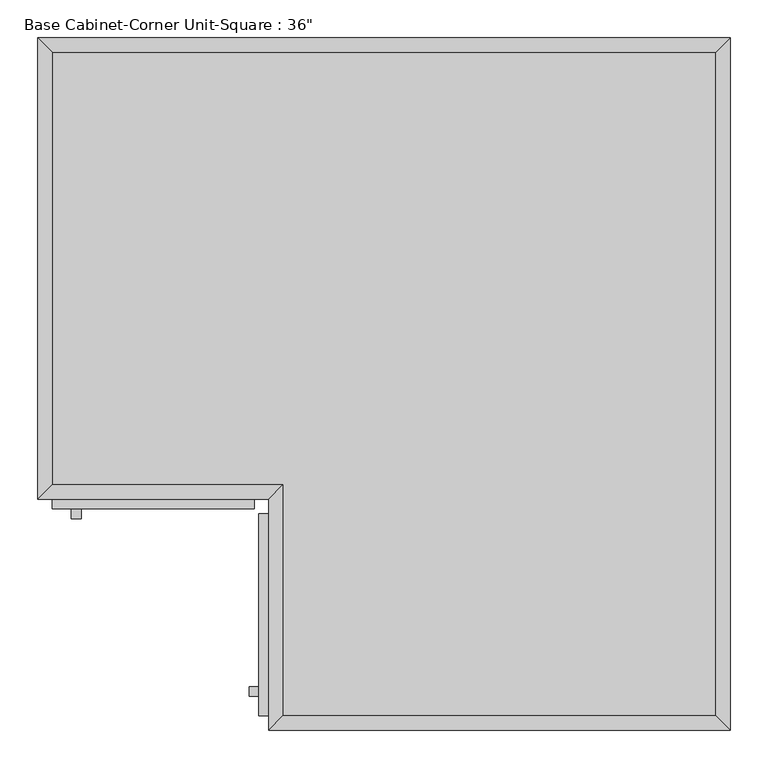
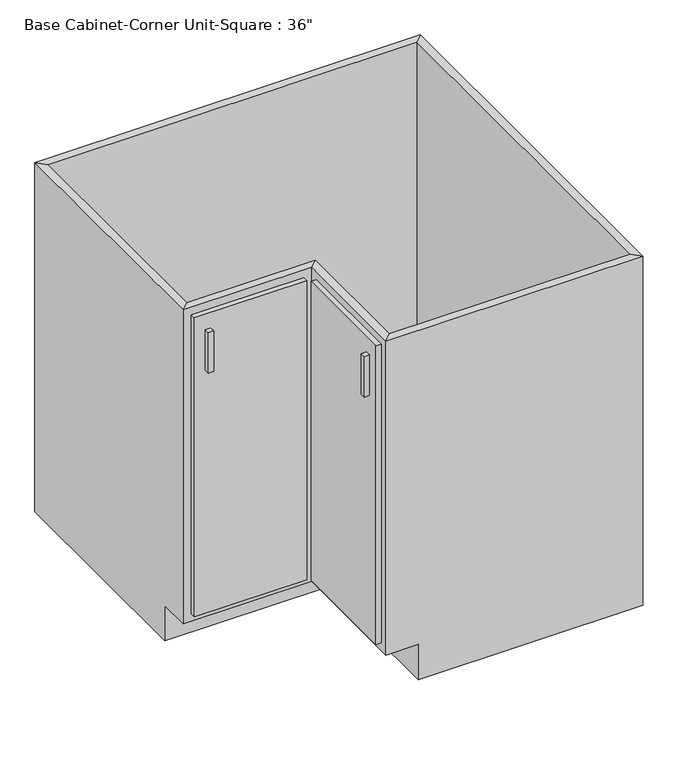
"""IFC4 building model written with IfcOpenShell, lengths in millimetres: furniture geometry."""

from ifc_helpers import new_model, si_unit, frame, origin, place, context, project, spatial, polyline, outline, extrude, faceted_brep, source, transform, mapped, element, save


def furniture_97fe820d(model_context):
    return source(origin(), model_context, "Body", "SolidModel", [
        extrude(outline(polyline([(507.6877049, -19.05), (507.6877049, -895.35), (-63.8122951, -895.35), (-63.8122951, -590.55), (-368.6122951, -590.55), (-368.6122951, -19.05), (507.6877049, -19.05)])), frame((0.0, 0.0, 88.9), z_axis=(0.0, 0.0, 1.0), x_axis=(1.0, 0.0, 0.0)), (0.0, 0.0, 1.0), 19.05),
        extrude(outline(polyline([(-101.9122951, -622.3), (-368.6122951, -622.3), (-368.6122951, -609.6), (-101.9122951, -609.6), (-101.9122951, -622.3)])), frame((0.0, 0.0, 107.95), z_axis=(0.0, 0.0, 1.0), x_axis=(1.0, 0.0, 0.0)), (0.0, 0.0, 1.0), 749.3),
        extrude(outline(polyline([(-330.5122951, -635.0), (-343.2122951, -635.0), (-343.2122951, -622.3), (-330.5122951, -622.3), (-330.5122951, -635.0)])), frame((0.0, 0.0, 717.55), z_axis=(0.0, 0.0, 1.0), x_axis=(1.0, 0.0, 0.0)), (0.0, 0.0, 1.0), 101.6),
        extrude(outline(polyline([(-82.8622951, -628.65), (-82.8622951, -895.35), (-95.5622951, -895.35), (-95.5622951, -628.65), (-82.8622951, -628.65)])), frame((0.0, 0.0, 107.95), z_axis=(0.0, 0.0, 1.0), x_axis=(1.0, 0.0, 0.0)), (0.0, 0.0, 1.0), 749.3),
        extrude(outline(polyline([(-95.5622951, -857.25), (-95.5622951, -869.95), (-108.2622951, -869.95), (-108.2622951, -857.25), (-95.5622951, -857.25)])), frame((0.0, 0.0, 717.55), z_axis=(0.0, 0.0, 1.0), x_axis=(1.0, 0.0, 0.0)), (0.0, 0.0, 1.0), 101.6),
        faceted_brep([(-368.6122951, -533.4, 88.9), (-6.6622951, -533.4, 88.9), (-6.6622951, -895.35, 88.9), (507.6877049, -895.35, 88.9), (507.6877049, -19.05, 88.9), (-368.6122951, -19.05, 88.9), (526.7377049, 0.0, 0.0), (526.7377049, -914.4, 0.0), (-6.6622951, -914.4, 0.0), (-6.6622951, -533.4, 0.0), (-387.6622951, -533.4, 0.0), (-387.6622951, 0.0, 0.0), (-387.6622951, 0.0, 876.3), (526.7377049, 0.0, 876.3), (-387.6622951, -533.4, 88.9), (-387.6622951, -609.6, 88.9), (-387.6622951, -609.6, 876.3), (-6.6622951, -914.4, 88.9), (526.7377049, -914.4, 876.3), (-82.8622951, -914.4, 876.3), (-82.8622951, -914.4, 88.9), (507.6877049, -895.35, 876.3), (-63.8122951, -895.35, 88.9), (-63.8122951, -895.35, 876.3), (-63.8122951, -590.55, 88.9), (-63.8122951, -590.55, 876.3), (-82.8622951, -609.6, 876.3), (-82.8622951, -609.6, 88.9), (-368.6122951, -590.55, 88.9), (-368.6122951, -590.55, 876.3), (-368.6122951, -19.05, 876.3), (507.6877049, -19.05, 876.3)], [[[0, 1, 2, 3, 4, 5]], [[6, 7, 8, 9, 10, 11]], [[6, 11, 12, 13]], [[12, 11, 10, 14, 15, 16]], [[10, 9, 1, 0, 14]], [[9, 8, 17, 2, 1]], [[8, 7, 18, 19, 20, 17]], [[18, 7, 6, 13]], [[21, 3, 2, 22, 23]], [[21, 23, 19, 18]], [[20, 22, 2, 17]], [[23, 22, 24, 25]], [[19, 23, 25, 26]], [[20, 19, 26, 27]], [[22, 20, 27, 24]], [[25, 24, 28, 29]], [[26, 25, 29, 16]], [[27, 26, 16, 15]], [[24, 27, 15, 28]], [[29, 28, 0, 5, 30]], [[16, 29, 30, 12]], [[28, 15, 14, 0]], [[30, 5, 4, 31]], [[12, 30, 31, 13]], [[3, 21, 31, 4]], [[21, 18, 13, 31]]]),
    ])


if __name__ == "__main__":
    model = new_model("IFC4")
    model_context = context("Model", 3, world=origin())
    ifc_project = project(units=[si_unit("LENGTHUNIT", "METRE", prefix="MILLI")], contexts=[model_context])
    site = spatial("IfcSite", under=ifc_project)
    building = spatial("IfcBuilding", under=site)
    placement = place(None, origin())
    furniture_shape = furniture_97fe820d(model_context)
    element("IfcFurniture", 1, ObjectType="Base Cabinet-Corner Unit-Square : 36\"", at=placement, inside=building, context=model_context, shape_type="MappedRepresentation", body=[
        mapped(furniture_shape, transform((0.0, 0.0, 0.0), x_axis=(1.0, 0.0, 0.0), y_axis=(0.0, 1.0, 0.0), z_axis=(0.0, 0.0, 1.0))),
    ])
    save(model, "model.ifc")

# Revit data of these elements
# Type "Base Cabinet-Corner Unit-Square : 36\""
#   Assembly Code = "C1030410"
#   Depth = 2 ft
#   Height = 2.875 ft
#   Toe Depth = 0.25 ft
#   Toe Height = 0.291667 ft
#   Width = 3 ft
#   Cabinet Material = Cabinets
#   Door/Drawer Material = Cabinets
#   Handle Material = Cabinets - Handles
#   Default Elevation = 0
# Element 1 (IfcFurniture, "Base Cabinet-Corner Unit-Square : 36\"")
#   Materials on its faces: "Cabinets", "Cabinets - Handles"
# Materials
#   "Cabinets": colour RGB 249 249 249, transparency 0
#   "Cabinets - Handles": colour RGB 57 57 57, transparency 0
